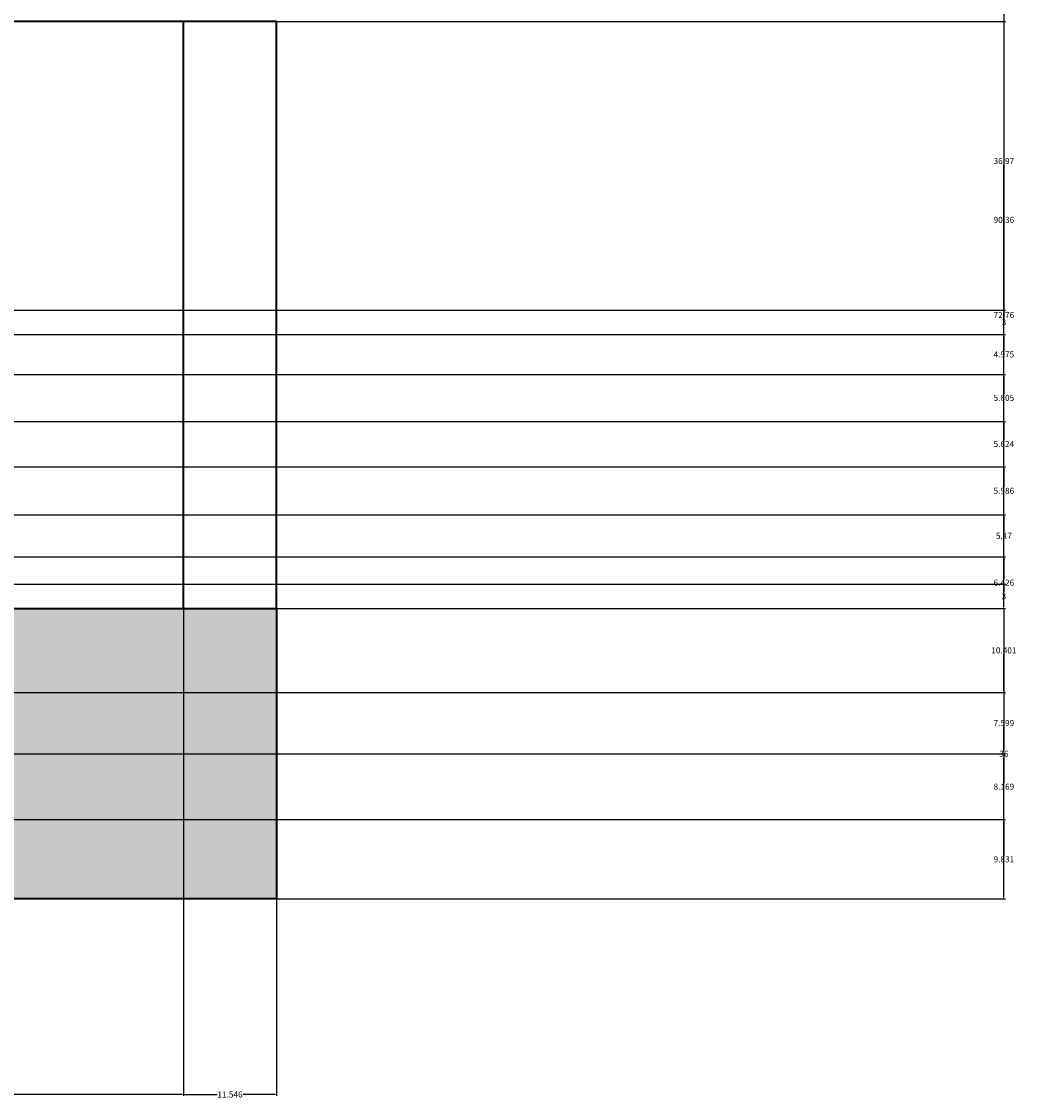
# Model space of a CAD drawing. Units: inches. Extents: x 62 to 566, y 66 to 528.
# Tile 14 of 20: x 443 to 566, y 66 to 199. Entities that reach past the tile are written whole.
import ezdxf

# ---------------------------------------------------------------- set-up
doc = ezdxf.new("R2010")
doc.units = ezdxf.units.IN
doc.header["$MEASUREMENT"] = 0
for name, color, linetype, lineweight in [('A-ANNO-DIMS', 2, 'Continuous', 18), ('A-ELEV', 7, 'Continuous', 35), ('A-WALL-PATT', 8, 'Continuous', 13)]:
    doc.layers.add(name, color=color, linetype=linetype, lineweight=lineweight)
doc.styles.get("Standard").update_dxf_attribs({"font": 'arial.ttf'})
doc.dimstyles.get("Standard").update_dxf_attribs({"dimtxt": 0.75, "dimasz": 0.18, "dimexe": 0.18, "dimexo": 0.0625, "dimgap": 0.09, "dimtad": 0, "dimtih": 1, "dimtoh": 1, "dimdec": 4, "dimzin": 0, "dimdsep": 46, "dimlunit": 4, "dimtxsty": 'Standard', "dimcen": 0.09, "dimadec": 0, "dimazin": 0, "dimtfac": 1, "dimtdec": 4, "dimtofl": 0, "dimtmove": 0, "dimatfit": 3, "dimfxl": 1, "dimtolj": 1, "dimtzin": 0, "dimarcsym": 0})

# ---------------------------------------------------------------- blocks, each defined once
blk = doc.blocks.new('*D12')
at = {"layer": 'A-ANNO-DIMS', "color": 0, "lineweight": -2, "transparency": 16777216}
for p, q in [((409.43, 126.31), (409.43, 65.94)), ((462.58, 126.31), (462.58, 65.94)), ((409.61, 66.12), (434.65, 66.12)), ((462.4, 66.12), (437.36, 66.12))]:
    blk.add_line(p, q, dxfattribs=at)
at = {"layer": 'A-ANNO-DIMS', "color": 0, "transparency": 16777216}
for points in [[(409.61, 66.15), (409.61, 66.09), (409.43, 66.12)], [(462.4, 66.15), (462.4, 66.09), (462.58, 66.12)]]:
    blk.add_solid(points, dxfattribs=at)
at = {"layer": 'Defpoints', "color": 0, "transparency": 16777216}
for p in [(409.43, 126.37), (462.58, 126.37), (462.58, 66.12)]:
    blk.add_point(p, dxfattribs=at)
at = {"layer": 'A-ANNO-DIMS', "color": 0, "transparency": 16777216, "insert": (436, 66.12), "char_height": 0.75, "attachment_point": 5}
blk.add_mtext('\\A1;53.14', dxfattribs=at)
blk = doc.blocks.new('*D13')
at = {"layer": 'A-ANNO-DIMS', "color": 0, "lineweight": -2, "transparency": 16777216}
for p, q in [((462.58, 126.31), (462.58, 65.94)), ((474.12, 90.31), (474.12, 65.94)), ((462.76, 66.12), (466.74, 66.12)), ((473.94, 66.12), (469.96, 66.12))]:
    blk.add_line(p, q, dxfattribs=at)
at = {"layer": 'A-ANNO-DIMS', "color": 0, "transparency": 16777216}
for points in [[(462.76, 66.15), (462.76, 66.09), (462.58, 66.12)], [(473.94, 66.15), (473.94, 66.09), (474.12, 66.12)]]:
    blk.add_solid(points, dxfattribs=at)
at = {"layer": 'Defpoints', "color": 0, "transparency": 16777216}
for p in [(462.58, 126.37), (474.12, 90.37), (474.12, 66.12)]:
    blk.add_point(p, dxfattribs=at)
at = {"layer": 'A-ANNO-DIMS', "color": 0, "transparency": 16777216, "insert": (468.35, 66.12), "char_height": 0.75, "attachment_point": 5}
blk.add_mtext('\\A1;11.546', dxfattribs=at)
blk = doc.blocks.new('*D19')
at = {"layer": 'A-ANNO-DIMS', "color": 0, "lineweight": -2, "transparency": 16777216}
for p, q in [((474.18, 126.37), (564.47, 126.37)), ((564.29, 126.19), (564.29, 108.84)), ((564.29, 90.55), (564.29, 107.9)), ((474.18, 90.37), (564.47, 90.37))]:
    blk.add_line(p, q, dxfattribs=at)
at = {"layer": 'A-ANNO-DIMS', "color": 0, "transparency": 16777216}
for points in [[(564.26, 126.19), (564.32, 126.19), (564.29, 126.37)], [(564.26, 90.55), (564.32, 90.55), (564.29, 90.37)]]:
    blk.add_solid(points, dxfattribs=at)
at = {"layer": 'Defpoints', "color": 0, "transparency": 16777216}
for p in [(474.12, 126.37), (564.29, 126.37), (474.12, 90.37)]:
    blk.add_point(p, dxfattribs=at)
at = {"layer": 'A-ANNO-DIMS', "color": 0, "transparency": 16777216, "insert": (564.29, 108.37), "char_height": 0.75, "attachment_point": 5}
blk.add_mtext('\\A1;36', dxfattribs=at)
blk = doc.blocks.new('*D20')
at = {"layer": 'A-ANNO-DIMS', "color": 0, "lineweight": -2, "transparency": 16777216}
for p, q in [((474.18, 199.13), (564.47, 199.13)), ((564.29, 198.95), (564.29, 163.22)), ((564.29, 126.55), (564.29, 162.28)), ((474.18, 126.37), (564.47, 126.37))]:
    blk.add_line(p, q, dxfattribs=at)
at = {"layer": 'A-ANNO-DIMS', "color": 0, "transparency": 16777216}
for points in [[(564.26, 198.95), (564.32, 198.95), (564.29, 199.13)], [(564.26, 126.55), (564.32, 126.55), (564.29, 126.37)]]:
    blk.add_solid(points, dxfattribs=at)
at = {"layer": 'Defpoints', "color": 0, "transparency": 16777216}
for p in [(474.12, 199.13), (564.29, 199.13), (474.12, 126.37)]:
    blk.add_point(p, dxfattribs=at)
at = {"layer": 'A-ANNO-DIMS', "color": 0, "transparency": 16777216, "insert": (564.29, 162.75), "char_height": 0.75, "attachment_point": 5}
blk.add_mtext('\\A1;72.76', dxfattribs=at)
blk = doc.blocks.new('*D65')
at = {"layer": 'A-ANNO-DIMS', "color": 0, "lineweight": -2, "transparency": 16777216}
for p, q in [((396.5, 100.2), (564.47, 100.2)), ((564.29, 100.02), (564.29, 95.76)), ((564.29, 90.55), (564.29, 94.81)), ((396.5, 90.37), (564.47, 90.37))]:
    blk.add_line(p, q, dxfattribs=at)
at = {"layer": 'A-ANNO-DIMS', "color": 0, "transparency": 16777216}
for points in [[(564.26, 100.02), (564.32, 100.02), (564.29, 100.2)], [(564.26, 90.55), (564.32, 90.55), (564.29, 90.37)]]:
    blk.add_solid(points, dxfattribs=at)
at = {"layer": 'Defpoints', "color": 0, "transparency": 16777216}
for p in [(396.43, 100.2), (564.29, 100.2), (396.43, 90.37)]:
    blk.add_point(p, dxfattribs=at)
at = {"layer": 'A-ANNO-DIMS', "color": 0, "transparency": 16777216, "insert": (564.29, 95.28), "char_height": 0.75, "attachment_point": 5}
blk.add_mtext('\\A1;9.831', dxfattribs=at)
blk = doc.blocks.new('*D66')
at = {"layer": 'A-ANNO-DIMS', "color": 0, "lineweight": -2, "transparency": 16777216}
for p, q in [((396.5, 108.37), (564.47, 108.37)), ((564.29, 108.19), (564.29, 104.76)), ((564.29, 100.38), (564.29, 103.81)), ((396.5, 100.2), (564.47, 100.2))]:
    blk.add_line(p, q, dxfattribs=at)
at = {"layer": 'A-ANNO-DIMS', "color": 0, "transparency": 16777216}
for points in [[(564.26, 108.19), (564.32, 108.19), (564.29, 108.37)], [(564.26, 100.38), (564.32, 100.38), (564.29, 100.2)]]:
    blk.add_solid(points, dxfattribs=at)
at = {"layer": 'Defpoints', "color": 0, "transparency": 16777216}
for p in [(396.43, 108.37), (564.29, 108.37), (396.43, 100.2)]:
    blk.add_point(p, dxfattribs=at)
at = {"layer": 'A-ANNO-DIMS', "color": 0, "transparency": 16777216, "insert": (564.29, 104.28), "char_height": 0.75, "attachment_point": 5}
blk.add_mtext('\\A1;8.169', dxfattribs=at)
blk = doc.blocks.new('*D67')
at = {"layer": 'A-ANNO-DIMS', "color": 0, "lineweight": -2, "transparency": 16777216}
for p, q in [((396.5, 115.97), (564.47, 115.97)), ((564.29, 115.79), (564.29, 112.64)), ((564.29, 108.55), (564.29, 111.69)), ((396.5, 108.37), (564.47, 108.37))]:
    blk.add_line(p, q, dxfattribs=at)
at = {"layer": 'A-ANNO-DIMS', "color": 0, "transparency": 16777216}
for points in [[(564.26, 115.79), (564.32, 115.79), (564.29, 115.97)], [(564.26, 108.55), (564.32, 108.55), (564.29, 108.37)]]:
    blk.add_solid(points, dxfattribs=at)
at = {"layer": 'Defpoints', "color": 0, "transparency": 16777216}
for p in [(396.43, 115.97), (564.29, 115.97), (396.43, 108.37)]:
    blk.add_point(p, dxfattribs=at)
at = {"layer": 'A-ANNO-DIMS', "color": 0, "transparency": 16777216, "insert": (564.29, 112.17), "char_height": 0.75, "attachment_point": 5}
blk.add_mtext('\\A1;7.599', dxfattribs=at)
blk = doc.blocks.new('*D68')
at = {"layer": 'A-ANNO-DIMS', "color": 0, "lineweight": -2, "transparency": 16777216}
for p, q in [((374.2, 126.37), (564.47, 126.37)), ((564.29, 126.19), (564.29, 121.64)), ((564.29, 116.15), (564.29, 120.69)), ((396.5, 115.97), (564.47, 115.97))]:
    blk.add_line(p, q, dxfattribs=at)
at = {"layer": 'A-ANNO-DIMS', "color": 0, "transparency": 16777216}
for points in [[(564.26, 126.19), (564.32, 126.19), (564.29, 126.37)], [(564.26, 116.15), (564.32, 116.15), (564.29, 115.97)]]:
    blk.add_solid(points, dxfattribs=at)
at = {"layer": 'Defpoints', "color": 0, "transparency": 16777216}
for p in [(374.14, 126.37), (564.29, 126.37), (396.43, 115.97)]:
    blk.add_point(p, dxfattribs=at)
at = {"layer": 'A-ANNO-DIMS', "color": 0, "transparency": 16777216, "insert": (564.29, 121.17), "char_height": 0.75, "attachment_point": 5}
blk.add_mtext('\\A1;10.401', dxfattribs=at)
blk = doc.blocks.new('*D69')
at = {"layer": 'A-ANNO-DIMS', "color": 0, "lineweight": -2, "transparency": 16777216}
for p, q in [((371.2, 129.37), (564.47, 129.37)), ((564.29, 129.19), (564.29, 128.34)), ((564.29, 126.55), (564.29, 127.4)), ((374.2, 126.37), (564.47, 126.37))]:
    blk.add_line(p, q, dxfattribs=at)
at = {"layer": 'A-ANNO-DIMS', "color": 0, "transparency": 16777216}
for points in [[(564.26, 129.19), (564.32, 129.19), (564.29, 129.37)], [(564.26, 126.55), (564.32, 126.55), (564.29, 126.37)]]:
    blk.add_solid(points, dxfattribs=at)
at = {"layer": 'Defpoints', "color": 0, "transparency": 16777216}
for p in [(371.14, 129.37), (564.29, 129.37), (374.14, 126.37)]:
    blk.add_point(p, dxfattribs=at)
at = {"layer": 'A-ANNO-DIMS', "color": 0, "transparency": 16777216, "insert": (564.29, 127.87), "char_height": 0.75, "attachment_point": 5}
blk.add_mtext('\\A1;3', dxfattribs=at)
blk = doc.blocks.new('*D70')
at = {"layer": 'A-ANNO-DIMS', "color": 0, "lineweight": -2, "transparency": 16777216}
for p, q in [((329.73, 219.73), (564.47, 219.73)), ((564.29, 219.55), (564.29, 175.02)), ((564.29, 129.55), (564.29, 174.08)), ((371.2, 129.37), (564.47, 129.37))]:
    blk.add_line(p, q, dxfattribs=at)
at = {"layer": 'A-ANNO-DIMS', "color": 0, "transparency": 16777216}
for points in [[(564.26, 219.55), (564.32, 219.55), (564.29, 219.73)], [(564.26, 129.55), (564.32, 129.55), (564.29, 129.37)]]:
    blk.add_solid(points, dxfattribs=at)
at = {"layer": 'Defpoints', "color": 0, "transparency": 16777216}
for p in [(329.67, 219.73), (564.29, 219.73), (371.14, 129.37)]:
    blk.add_point(p, dxfattribs=at)
at = {"layer": 'A-ANNO-DIMS', "color": 0, "transparency": 16777216, "insert": (564.29, 174.55), "char_height": 0.75, "attachment_point": 5}
blk.add_mtext('\\A1;90.36', dxfattribs=at)
blk = doc.blocks.new('*D116')
at = {"layer": 'A-ANNO-DIMS', "color": 0, "lineweight": -2, "transparency": 16777216}
for p, q in [((267.86, 132.79), (564.47, 132.79)), ((564.29, 132.61), (564.29, 130.05)), ((564.29, 126.55), (564.29, 129.11)), ((272.12, 126.37), (564.47, 126.37))]:
    blk.add_line(p, q, dxfattribs=at)
at = {"layer": 'A-ANNO-DIMS', "color": 0, "transparency": 16777216}
for points in [[(564.26, 132.61), (564.32, 132.61), (564.29, 132.79)], [(564.26, 126.55), (564.32, 126.55), (564.29, 126.37)]]:
    blk.add_solid(points, dxfattribs=at)
at = {"layer": 'Defpoints', "color": 0, "transparency": 16777216}
for p in [(267.79, 132.79), (564.29, 132.79), (272.06, 126.37)]:
    blk.add_point(p, dxfattribs=at)
at = {"layer": 'A-ANNO-DIMS', "color": 0, "transparency": 16777216, "insert": (564.29, 129.58), "char_height": 0.75, "attachment_point": 5}
blk.add_mtext('\\A1;6.426', dxfattribs=at)
blk = doc.blocks.new('*D117')
at = {"layer": 'A-ANNO-DIMS', "color": 0, "lineweight": -2, "transparency": 16777216}
for p, q in [((267.86, 137.96), (564.47, 137.96)), ((564.29, 137.78), (564.29, 135.85)), ((564.29, 132.97), (564.29, 134.91)), ((267.86, 132.79), (564.47, 132.79))]:
    blk.add_line(p, q, dxfattribs=at)
at = {"layer": 'A-ANNO-DIMS', "color": 0, "transparency": 16777216}
for points in [[(564.26, 137.78), (564.32, 137.78), (564.29, 137.96)], [(564.26, 132.97), (564.32, 132.97), (564.29, 132.79)]]:
    blk.add_solid(points, dxfattribs=at)
at = {"layer": 'Defpoints', "color": 0, "transparency": 16777216}
for p in [(267.79, 137.96), (564.29, 137.96), (267.79, 132.79)]:
    blk.add_point(p, dxfattribs=at)
at = {"layer": 'A-ANNO-DIMS', "color": 0, "transparency": 16777216, "insert": (564.29, 135.38), "char_height": 0.75, "attachment_point": 5}
blk.add_mtext('\\A1;5.17', dxfattribs=at)
blk = doc.blocks.new('*D118')
at = {"layer": 'A-ANNO-DIMS', "color": 0, "lineweight": -2, "transparency": 16777216}
for p, q in [((267.86, 143.95), (564.47, 143.95)), ((564.29, 143.77), (564.29, 141.43)), ((564.29, 138.14), (564.29, 140.49)), ((267.86, 137.96), (564.47, 137.96))]:
    blk.add_line(p, q, dxfattribs=at)
at = {"layer": 'A-ANNO-DIMS', "color": 0, "transparency": 16777216}
for points in [[(564.26, 143.77), (564.32, 143.77), (564.29, 143.95)], [(564.26, 138.14), (564.32, 138.14), (564.29, 137.96)]]:
    blk.add_solid(points, dxfattribs=at)
at = {"layer": 'Defpoints', "color": 0, "transparency": 16777216}
for p in [(267.79, 143.95), (564.29, 143.95), (267.79, 137.96)]:
    blk.add_point(p, dxfattribs=at)
at = {"layer": 'A-ANNO-DIMS', "color": 0, "transparency": 16777216, "insert": (564.29, 140.96), "char_height": 0.75, "attachment_point": 5}
blk.add_mtext('\\A1;5.986', dxfattribs=at)
blk = doc.blocks.new('*D119')
at = {"layer": 'A-ANNO-DIMS', "color": 0, "lineweight": -2, "transparency": 16777216}
for p, q in [((267.86, 149.57), (564.47, 149.57)), ((564.29, 149.39), (564.29, 147.24)), ((564.29, 144.13), (564.29, 146.29)), ((267.86, 143.95), (564.47, 143.95))]:
    blk.add_line(p, q, dxfattribs=at)
at = {"layer": 'A-ANNO-DIMS', "color": 0, "transparency": 16777216}
for points in [[(564.26, 149.39), (564.32, 149.39), (564.29, 149.57)], [(564.26, 144.13), (564.32, 144.13), (564.29, 143.95)]]:
    blk.add_solid(points, dxfattribs=at)
at = {"layer": 'Defpoints', "color": 0, "transparency": 16777216}
for p in [(267.79, 149.57), (564.29, 149.57), (267.79, 143.95)]:
    blk.add_point(p, dxfattribs=at)
at = {"layer": 'A-ANNO-DIMS', "color": 0, "transparency": 16777216, "insert": (564.29, 146.76), "char_height": 0.75, "attachment_point": 5}
blk.add_mtext('\\A1;5.624', dxfattribs=at)
blk = doc.blocks.new('*D120')
at = {"layer": 'A-ANNO-DIMS', "color": 0, "lineweight": -2, "transparency": 16777216}
for p, q in [((267.86, 155.38), (564.47, 155.38)), ((564.29, 155.2), (564.29, 152.95)), ((564.29, 149.75), (564.29, 152)), ((267.86, 149.57), (564.47, 149.57))]:
    blk.add_line(p, q, dxfattribs=at)
at = {"layer": 'A-ANNO-DIMS', "color": 0, "transparency": 16777216}
for points in [[(564.26, 155.2), (564.32, 155.2), (564.29, 155.38)], [(564.26, 149.75), (564.32, 149.75), (564.29, 149.57)]]:
    blk.add_solid(points, dxfattribs=at)
at = {"layer": 'Defpoints', "color": 0, "transparency": 16777216}
for p in [(267.79, 155.38), (564.29, 155.38), (267.79, 149.57)]:
    blk.add_point(p, dxfattribs=at)
at = {"layer": 'A-ANNO-DIMS', "color": 0, "transparency": 16777216, "insert": (564.29, 152.48), "char_height": 0.75, "attachment_point": 5}
blk.add_mtext('\\A1;5.805', dxfattribs=at)
blk = doc.blocks.new('*D121')
at = {"layer": 'A-ANNO-DIMS', "color": 0, "lineweight": -2, "transparency": 16777216}
for p, q in [((272.12, 160.35), (564.47, 160.35)), ((564.29, 160.17), (564.29, 158.34)), ((564.29, 155.56), (564.29, 157.39)), ((267.86, 155.38), (564.47, 155.38))]:
    blk.add_line(p, q, dxfattribs=at)
at = {"layer": 'A-ANNO-DIMS', "color": 0, "transparency": 16777216}
for points in [[(564.26, 160.17), (564.32, 160.17), (564.29, 160.35)], [(564.26, 155.56), (564.32, 155.56), (564.29, 155.38)]]:
    blk.add_solid(points, dxfattribs=at)
at = {"layer": 'Defpoints', "color": 0, "transparency": 16777216}
for p in [(272.06, 160.35), (564.29, 160.35), (267.79, 155.38)]:
    blk.add_point(p, dxfattribs=at)
at = {"layer": 'A-ANNO-DIMS', "color": 0, "transparency": 16777216, "insert": (564.29, 157.87), "char_height": 0.75, "attachment_point": 5}
blk.add_mtext('\\A1;4.975', dxfattribs=at)
blk = doc.blocks.new('*D122')
at = {"layer": 'A-ANNO-DIMS', "color": 0, "lineweight": -2, "transparency": 16777216}
for p, q in [((269.12, 163.35), (564.47, 163.35)), ((564.29, 163.17), (564.29, 162.33)), ((272.12, 160.35), (564.47, 160.35)), ((564.29, 160.53), (564.29, 161.38))]:
    blk.add_line(p, q, dxfattribs=at)
at = {"layer": 'A-ANNO-DIMS', "color": 0, "transparency": 16777216}
for points in [[(564.26, 163.17), (564.32, 163.17), (564.29, 163.35)], [(564.26, 160.53), (564.32, 160.53), (564.29, 160.35)]]:
    blk.add_solid(points, dxfattribs=at)
at = {"layer": 'Defpoints', "color": 0, "transparency": 16777216}
for p in [(269.06, 163.35), (564.29, 163.35), (272.06, 160.35)]:
    blk.add_point(p, dxfattribs=at)
at = {"layer": 'A-ANNO-DIMS', "color": 0, "transparency": 16777216, "insert": (564.29, 161.85), "char_height": 0.75, "attachment_point": 5}
blk.add_mtext('\\A1;3', dxfattribs=at)
blk = doc.blocks.new('*D123')
at = {"layer": 'A-ANNO-DIMS', "color": 0, "lineweight": -2, "transparency": 16777216}
for p, q in [((269.12, 200.32), (564.47, 200.32)), ((564.29, 200.14), (564.29, 182.31)), ((564.29, 163.53), (564.29, 181.37)), ((269.12, 163.35), (564.47, 163.35))]:
    blk.add_line(p, q, dxfattribs=at)
at = {"layer": 'A-ANNO-DIMS', "color": 0, "transparency": 16777216}
for points in [[(564.26, 200.14), (564.32, 200.14), (564.29, 200.32)], [(564.26, 163.53), (564.32, 163.53), (564.29, 163.35)]]:
    blk.add_solid(points, dxfattribs=at)
at = {"layer": 'Defpoints', "color": 0, "transparency": 16777216}
for p in [(269.06, 200.32), (564.29, 200.32), (269.06, 163.35)]:
    blk.add_point(p, dxfattribs=at)
at = {"layer": 'A-ANNO-DIMS', "color": 0, "transparency": 16777216, "insert": (564.29, 181.84), "char_height": 0.75, "attachment_point": 5}
blk.add_mtext('\\A1;36.97', dxfattribs=at)

msp = doc.modelspace()

# ---------------------------------------------------------------- hatches: boundary and pattern name
at = {"layer": 'A-WALL-PATT'}
h = msp.add_hatch(dxfattribs=at)
h.set_pattern_fill('ANSI36', color=256, scale=8.8)
h.paths.add_polyline_path([(217.2752, 420.597), (169.0431, 420.597), (169.0431, 126.3686), (217.2752, 126.3686), (217.2752, 129.0504), (217.2752, 271.4128), (217.2752, 295.4128), (217.2752, 307.4128)])
h.paths.add_polyline_path([(282.3509, 501.0423), (125.9418, 501.0423), (125.9418, 465.0423), (282.3509, 465.0423)])
h.paths.add_polyline_path([(209.709, 476.6506), (202.045, 476.6506), (202.045, 493.7764), (209.709, 493.7764)], flags=16)
h.paths.add_polyline_path([(193.9913, 476.6506), (186.3273, 476.6506), (186.3273, 493.7764), (193.9913, 493.7764)], flags=16)
h.paths.add_polyline_path([(177.9243, 476.6506), (170.2603, 476.6506), (170.2603, 493.7764), (177.9243, 493.7764)], flags=16)
h.paths.add_polyline_path([(163.2545, 476.3015), (155.5905, 476.3015), (155.5905, 493.4274), (163.2545, 493.4274)], flags=16)
h.paths.add_polyline_path([(148.2354, 476.3015), (140.5713, 476.3015), (140.5713, 493.4274), (148.2354, 493.4274)], flags=16)
h.paths.add_polyline_path([(284.2021, 126.3686), (87.8962, 126.3686), (87.8962, 114.3686), (87.8962, 90.3686), (284.2021, 90.3686)])
h.paths.add_polyline_path([(474.1214, 126.3686), (396.433, 126.3686), (396.433, 90.3686), (474.1214, 90.3686)])

# ---------------------------------------------------------------- linework, layer by layer
at = {"layer": 'A-ELEV'}
for p, q in [((474.1214, 199.1332), (409.433, 199.1332)), ((462.5753, 126.3686), (462.5753, 199.1332)), ((474.1214, 126.3686), (474.1214, 199.1332)), ((396.433, 126.3686), (474.1214, 126.3686)), ((474.1214, 126.3686), (474.1214, 90.3686)), ((474.1214, 90.3686), (396.433, 90.3686))]:
    msp.add_line(p, q, dxfattribs=at)

# ---------------------------------------------------------------- dimensions: what is measured, and where the dimension line sits
at = {"layer": 'A-ANNO-DIMS'}
for base, p1, p2, override, picture, middle in [((564.2868, 219.7304), (371.1373, 129.3686), (329.6665, 219.7304), {"dimdec": 2, "dimlfac": 1, "dimrnd": 0, "dimzin": 0, "dimdsep": 46, "dimlunit": 2}, '*D70', (564.2868, 174.5495)), ((564.2868, 200.3236), (269.0586, 163.3545), (269.0586, 200.3236), {"dimdec": 2, "dimlfac": 1, "dimrnd": 0, "dimzin": 0, "dimdsep": 46, "dimlunit": 2}, '*D123', (564.2868, 181.8391)), ((564.2868, 199.1332), (474.1214, 126.3686), (474.1214, 199.1332), {"dimdec": 2, "dimlfac": 1, "dimrnd": 0, "dimzin": 0, "dimdsep": 46, "dimlunit": 2}, '*D20', (564.2868, 162.7509)), ((564.2868, 163.3545), (272.0586, 160.3545), (269.0586, 163.3545), {"dimdec": 0, "dimlfac": 1, "dimrnd": 0, "dimzin": 0, "dimdsep": 46, "dimlunit": 2}, '*D122', (564.2868, 161.8545)), ((564.2868, 160.3545), (267.7931, 155.3799), (272.0586, 160.3545), {"dimdec": 3, "dimlfac": 1, "dimrnd": 0, "dimzin": 0, "dimdsep": 46, "dimlunit": 2}, '*D121', (564.2868, 157.8672)), ((564.2868, 155.3799), (267.7931, 149.5749), (267.7931, 155.3799), {"dimdec": 3, "dimlfac": 1, "dimrnd": 0, "dimzin": 0, "dimdsep": 46, "dimlunit": 2}, '*D120', (564.2868, 152.4774)), ((564.2868, 149.5749), (267.7931, 143.9513), (267.7931, 149.5749), {"dimdec": 3, "dimlfac": 1, "dimrnd": 0, "dimzin": 0, "dimdsep": 46, "dimlunit": 2}, '*D119', (564.2868, 146.7631)), ((564.2868, 143.9513), (267.7931, 137.9649), (267.7931, 143.9513), {"dimdec": 3, "dimlfac": 1, "dimrnd": 0, "dimzin": 0, "dimdsep": 46, "dimlunit": 2}, '*D118', (564.2868, 140.9581)), ((564.2868, 137.9649), (267.7931, 132.7949), (267.7931, 137.9649), {"dimdec": 2, "dimlfac": 1, "dimrnd": 0, "dimzin": 0, "dimdsep": 46, "dimlunit": 2}, '*D117', (564.2868, 135.3799)), ((564.2868, 132.7949), (272.0586, 126.3686), (267.7931, 132.7949), {"dimdec": 3, "dimlfac": 1, "dimrnd": 0, "dimzin": 0, "dimdsep": 46, "dimlunit": 2}, '*D116', (564.2868, 129.5817)), ((564.2868, 129.3686), (374.1373, 126.3686), (371.1373, 129.3686), {"dimdec": 0, "dimlfac": 1, "dimrnd": 0, "dimzin": 0, "dimdsep": 46, "dimlunit": 2}, '*D69', (564.2868, 127.8686)), ((564.2868, 126.3686), (396.433, 115.9672), (374.1373, 126.3686), {"dimdec": 3, "dimlfac": 1, "dimrnd": 0, "dimzin": 0, "dimdsep": 46, "dimlunit": 2}, '*D68', (564.2868, 121.1679)), ((564.2868, 126.3686), (474.1214, 90.3686), (474.1214, 126.3686), {"dimdec": 0, "dimlfac": 1, "dimrnd": 0, "dimzin": 0, "dimdsep": 46, "dimlunit": 2}, '*D19', (564.2868, 108.3686)), ((564.2868, 115.9672), (396.433, 108.3686), (396.433, 115.9672), {"dimdec": 3, "dimlfac": 1, "dimrnd": 0, "dimzin": 0, "dimdsep": 46, "dimlunit": 2}, '*D67', (564.2868, 112.1679)), ((564.2868, 108.3686), (396.433, 100.1998), (396.433, 108.3686), {"dimdec": 3, "dimlfac": 1, "dimrnd": 0, "dimzin": 0, "dimdsep": 46, "dimlunit": 2}, '*D66', (564.2868, 104.2842)), ((564.2868, 100.1998), (396.433, 90.3686), (396.433, 100.1998), {"dimdec": 3, "dimlfac": 1, "dimrnd": 0, "dimzin": 0, "dimdsep": 46, "dimlunit": 2}, '*D65', (564.2868, 95.2842))]:
    dim = msp.add_linear_dim(base=base, p1=p1, p2=p2, angle=90, dimstyle='Standard', override=override, dxfattribs=at)
    dim.commit()
    dim.dimension.update_dxf_attribs({"geometry": picture, "text_midpoint": middle})
for base, p1, p2, override, picture, middle in [((462.5753, 66.1186), (409.433, 126.3686), (462.5753, 126.3686), {"dimdec": 2, "dimlfac": 1, "dimrnd": 0, "dimzin": 0, "dimdsep": 46, "dimlunit": 2}, '*D12', (436.0042, 66.1186)), ((474.1214, 66.1186), (462.5753, 126.3686), (474.1214, 90.3686), {"dimdec": 3, "dimlfac": 1, "dimrnd": 0, "dimzin": 0, "dimdsep": 46, "dimlunit": 2}, '*D13', (468.3483, 66.1186))]:
    dim = msp.add_linear_dim(base=base, p1=p1, p2=p2, dimstyle='Standard', override=override, dxfattribs=at)
    dim.commit()
    dim.dimension.update_dxf_attribs({"geometry": picture, "text_midpoint": middle})

doc.saveas('drawing.dxf')
